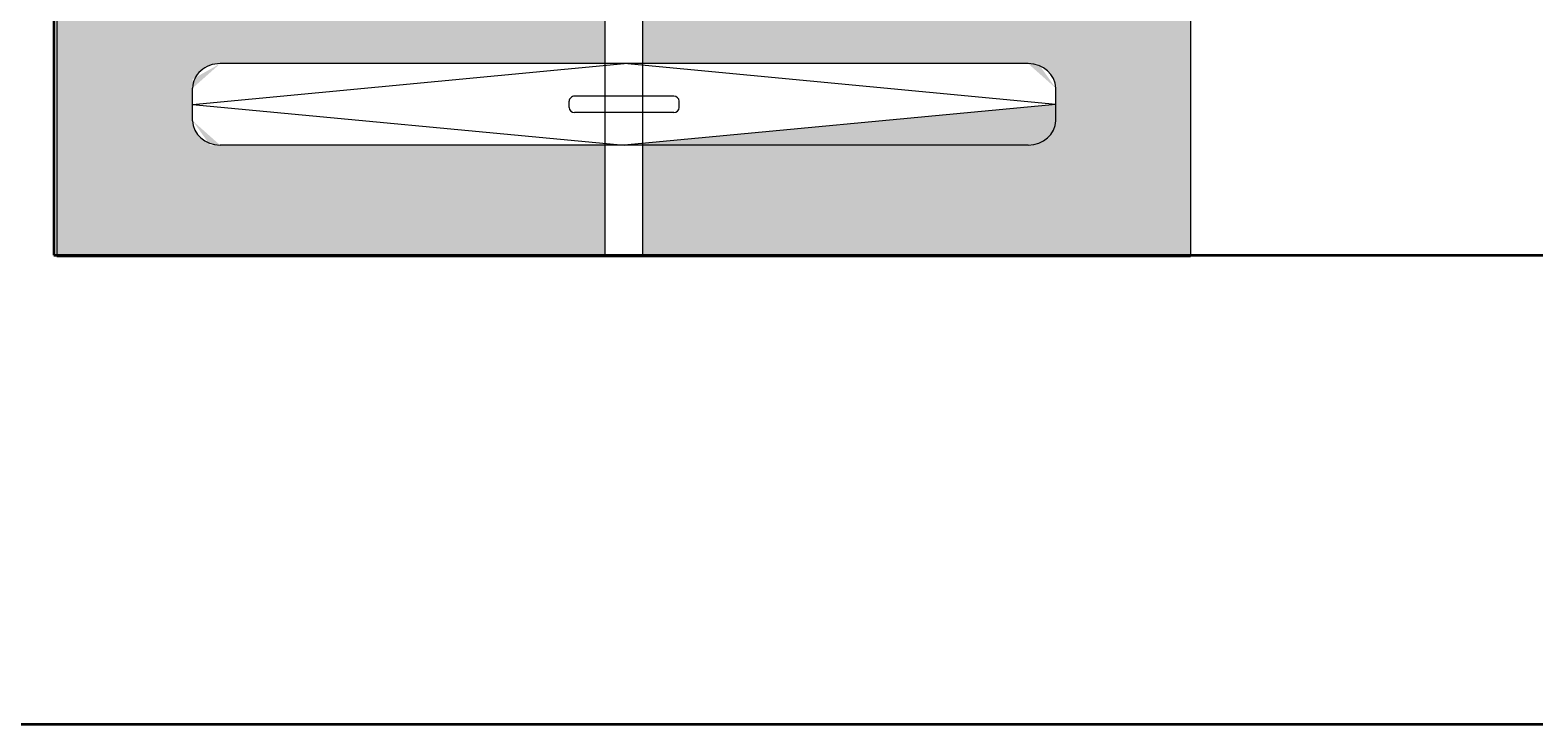
# Model space of a CAD drawing. Units: millimetres. Extents: x 27017497 to 27018854, y 7058029 to 7059154.
# Tile 5 of 91: x 27017622 to 27017651, y 7058133 to 7058146. Entities that reach past the tile are written whole.
import ezdxf

# ---------------------------------------------------------------- set-up
doc = ezdxf.new("R2010")
doc.units = ezdxf.units.MM
for name, color, linetype, lineweight in [('A-ANNO-DIMS', 2, 'Continuous', 18), ('A-FLOR-CASE', 8, 'Continuous', 20), ('A-FLOR-CASE-PATT', 44, 'Continuous', 13), ('A-WALL', 7, 'Continuous', 35)]:
    doc.layers.add(name, color=color, linetype=linetype, lineweight=lineweight)
doc.styles.get("Standard").update_dxf_attribs({"font": 'arial.ttf'})
doc.dimstyles.get("Standard").update_dxf_attribs({"dimtxt": 0.18, "dimasz": 0.18, "dimexe": 0.18, "dimexo": 0.0625, "dimgap": 0.09, "dimtad": 0, "dimtih": 1, "dimtoh": 1, "dimdec": 4, "dimzin": 0, "dimdsep": 46, "dimtxsty": 'Standard', "dimcen": 0.09, "dimadec": 0, "dimazin": 0, "dimtfac": 1, "dimtdec": 4, "dimtofl": 0, "dimtmove": 0, "dimatfit": 3, "dimfxl": 1, "dimtolj": 1, "dimtzin": 0, "dimarcsym": 0})

# ---------------------------------------------------------------- blocks, each defined once
blk = doc.blocks.new('WARDROBE-HANGING')
for p, q in [((0, 21.737), (65.212, 21.737)), ((65.212, 0), (65.212, 21.737)), ((62.293, 19.153), (61.511, 10.877)), ((62.606, 19.153), (61.98, 19.153)), ((62.293, 19.153), (63.076, 10.877)), ((61.511, 18.624), (61.511, 3.13)), ((63.076, 18.624), (63.076, 3.13)), ((62.137, 11.828), (62.137, 9.927)), ((62.356, 11.934), (62.231, 11.934)), ((62.45, 11.828), (62.45, 9.927)), ((0, 11.231), (65.212, 11.231)), ((62.293, 2.602), (61.511, 10.877)), ((62.293, 2.602), (63.076, 10.877)), ((0, 10.506), (65.212, 10.506)), ((62.356, 9.821), (62.231, 9.821)), ((62.606, 2.602), (61.98, 2.602)), ((0, 0), (65.212, 0))]:
    blk.add_line(p, q)
for centre, major_axis, start_param, end_param in [((61.98, 18.624), (0, 0.528), 0, 1.570796), ((62.606, 18.624), (0, 0.528), 4.712389, 6.283185), ((62.231, 11.828), (0, 0.106), 0, 1.570796), ((62.356, 11.828), (0, 0.106), -1.570796, 0), ((62.231, 9.927), (0, 0.106), 1.570796, 3.141593), ((62.356, 9.927), (0, 0.106), 3.141593, 4.712389), ((61.98, 3.13), (0, 0.528), 1.570796, 3.141593), ((62.606, 3.13), (0, 0.528), 3.141593, 4.712389)]:
    blk.add_ellipse(centre, major_axis=major_axis, ratio=0.888892, start_param=start_param, end_param=end_param)
blk = doc.blocks.new('*D47')
at = {"layer": 'A-ANNO-DIMS', "color": 0, "lineweight": -2, "transparency": 16777216}
for p, q in [((27017561.166, 7058294.35), (27017561.166, 7058028.6)), ((27018790.606, 7058294.35), (27018790.606, 7058028.6)), ((27017561.346, 7058028.78), (27018175.431, 7058028.78)), ((27018790.426, 7058028.78), (27018176.341, 7058028.78))]:
    blk.add_line(p, q, dxfattribs=at)
at = {"layer": 'A-ANNO-DIMS', "color": 0, "transparency": 16777216}
for points in [[(27017561.346, 7058028.81), (27017561.346, 7058028.75), (27017561.166, 7058028.78)], [(27018790.426, 7058028.81), (27018790.426, 7058028.75), (27018790.606, 7058028.78)]]:
    blk.add_solid(points, dxfattribs=at)
at = {"layer": 'Defpoints', "color": 0, "transparency": 16777216}
for p in [(27017561.166, 7058294.412), (27018790.606, 7058294.412), (27018790.606, 7058028.78)]:
    blk.add_point(p, dxfattribs=at)
at = {"layer": 'A-ANNO-DIMS', "color": 0, "transparency": 16777216, "insert": (27018175.886, 7058028.78), "char_height": 0.18, "attachment_point": 5}
blk.add_mtext('\\A1;1229.4', dxfattribs=at)
blk = doc.blocks.new('*D48')
at = {"layer": 'A-ANNO-DIMS', "color": 0, "lineweight": -2, "transparency": 16777216}
for p, q in [((27018463.498, 7058622.912), (27017497.536, 7058622.912)), ((27017497.716, 7058622.732), (27017497.716, 7058357.753)), ((27017497.716, 7058092.41), (27017497.716, 7058357.389)), ((27018555.129, 7058092.23), (27017497.536, 7058092.23))]:
    blk.add_line(p, q, dxfattribs=at)
at = {"layer": 'A-ANNO-DIMS', "color": 0, "transparency": 16777216}
for points in [[(27017497.686, 7058622.732), (27017497.746, 7058622.732), (27017497.716, 7058622.912)], [(27017497.686, 7058092.41), (27017497.746, 7058092.41), (27017497.716, 7058092.23)]]:
    blk.add_solid(points, dxfattribs=at)
at = {"layer": 'Defpoints', "color": 0, "transparency": 16777216}
for p in [(27018463.561, 7058622.912), (27017497.716, 7058092.23), (27018555.192, 7058092.23)]:
    blk.add_point(p, dxfattribs=at)
at = {"layer": 'A-ANNO-DIMS', "color": 0, "transparency": 16777216, "insert": (27017497.716, 7058357.571), "char_height": 0.18, "attachment_point": 5}
blk.add_mtext('\\A1;530.7', dxfattribs=at)

msp = doc.modelspace()

# ---------------------------------------------------------------- hatches: boundary and pattern name
at = {"layer": 'A-FLOR-CASE-PATT'}
h = msp.add_hatch(color=256, dxfattribs=at)
h.dxf.hatch_style = 1
edge = h.paths.add_edge_path()
edge.add_line((27017644.461, 7058207.1), (27017639.716, 7058207.1))
edge.add_line((27017639.716, 7058207.1), (27017639.716, 7058207.055))
edge.add_line((27017639.716, 7058207.055), (27017633.955, 7058207.055))
edge.add_line((27017633.955, 7058207.055), (27017633.955, 7058203.02))
edge.add_line((27017633.955, 7058203.02), (27017641.542, 7058203.02))
edge.add_ellipse((27017641.349, 7058202.551), major_axis=(0.528, 0), ratio=0.888892, start_angle=0, end_angle=90, ccw=False)
edge.add_line((27017641.877, 7058202.551), (27017641.877, 7058202.238))
edge.add_line((27017641.877, 7058202.238), (27017633.955, 7058201.488))
edge.add_line((27017633.955, 7058201.488), (27017633.955, 7058199.747))
edge.add_line((27017633.955, 7058199.747), (27017641.542, 7058199.747))
edge.add_ellipse((27017641.349, 7058199.277), major_axis=(0.528, 0), ratio=0.888892, start_angle=0, end_angle=90, ccw=False)
edge.add_line((27017641.877, 7058199.277), (27017641.877, 7058198.964))
edge.add_line((27017641.877, 7058198.964), (27017633.955, 7058198.215))
edge.add_line((27017633.955, 7058198.215), (27017633.955, 7058193.415))
edge.add_line((27017633.955, 7058193.415), (27017641.403, 7058190.704))
edge.add_ellipse((27017641.06, 7058190.329), major_axis=(0.496, -0.181), ratio=0.888892, start_angle=0, end_angle=90, ccw=False)
edge.add_line((27017641.557, 7058190.148), (27017641.45, 7058189.854))
edge.add_line((27017641.45, 7058189.854), (27017633.955, 7058191.806))
edge.add_line((27017633.955, 7058191.806), (27017633.955, 7058188.22))
edge.add_line((27017633.955, 7058188.22), (27017641.542, 7058188.22))
edge.add_ellipse((27017641.349, 7058187.75), major_axis=(0.528, 0), ratio=0.888892, start_angle=0, end_angle=90, ccw=False)
edge.add_line((27017641.877, 7058187.75), (27017641.877, 7058187.437))
edge.add_line((27017641.877, 7058187.437), (27017633.955, 7058186.688))
edge.add_line((27017633.955, 7058186.688), (27017633.955, 7058181.982))
edge.add_line((27017633.955, 7058181.982), (27017641.542, 7058181.982))
edge.add_ellipse((27017641.349, 7058181.513), major_axis=(0.528, 0), ratio=0.888892, start_angle=0, end_angle=90, ccw=False)
edge.add_line((27017641.877, 7058181.513), (27017641.877, 7058181.199))
edge.add_line((27017641.877, 7058181.199), (27017633.955, 7058180.45))
edge.add_line((27017633.955, 7058180.45), (27017633.955, 7058178.709))
edge.add_line((27017633.955, 7058178.709), (27017641.542, 7058178.709))
edge.add_ellipse((27017641.349, 7058178.239), major_axis=(0.528, 0), ratio=0.888892, start_angle=0, end_angle=90, ccw=False)
edge.add_line((27017641.877, 7058178.239), (27017641.877, 7058177.926))
edge.add_line((27017641.877, 7058177.926), (27017633.955, 7058177.177))
edge.add_line((27017633.955, 7058177.177), (27017633.955, 7058173.878))
edge.add_line((27017633.955, 7058173.878), (27017641.403, 7058171.167))
edge.add_ellipse((27017641.06, 7058170.792), major_axis=(0.496, -0.181), ratio=0.888892, start_angle=0, end_angle=90, ccw=False)
edge.add_line((27017641.557, 7058170.611), (27017641.45, 7058170.317))
edge.add_line((27017641.45, 7058170.317), (27017633.955, 7058172.269))
edge.add_line((27017633.955, 7058172.269), (27017633.955, 7058168.293))
edge.add_line((27017633.955, 7058168.293), (27017641.542, 7058168.293))
edge.add_ellipse((27017641.349, 7058167.824), major_axis=(0.528, 0), ratio=0.888892, start_angle=0, end_angle=90, ccw=False)
edge.add_line((27017641.877, 7058167.824), (27017641.877, 7058167.511))
edge.add_line((27017641.877, 7058167.511), (27017633.955, 7058166.762))
edge.add_line((27017633.955, 7058166.762), (27017633.955, 7058160.389))
edge.add_line((27017633.955, 7058160.389), (27017641.542, 7058160.389))
edge.add_ellipse((27017641.349, 7058159.92), major_axis=(0.528, 0), ratio=0.888892, start_angle=0, end_angle=90, ccw=False)
edge.add_line((27017641.877, 7058159.92), (27017641.877, 7058159.607))
edge.add_line((27017641.877, 7058159.607), (27017633.955, 7058158.858))
edge.add_line((27017633.955, 7058158.858), (27017633.955, 7058157.116))
edge.add_line((27017633.955, 7058157.116), (27017641.542, 7058157.116))
edge.add_ellipse((27017641.349, 7058156.647), major_axis=(0.528, 0), ratio=0.888892, start_angle=0, end_angle=90, ccw=False)
edge.add_line((27017641.877, 7058156.647), (27017641.877, 7058156.334))
edge.add_line((27017641.877, 7058156.334), (27017633.955, 7058155.585))
edge.add_line((27017633.955, 7058155.585), (27017633.955, 7058150.784))
edge.add_line((27017633.955, 7058150.784), (27017641.403, 7058148.073))
edge.add_ellipse((27017641.06, 7058147.698), major_axis=(0.496, -0.181), ratio=0.888892, start_angle=0, end_angle=90, ccw=False)
edge.add_line((27017641.557, 7058147.517), (27017641.45, 7058147.223))
edge.add_line((27017641.45, 7058147.223), (27017633.955, 7058149.175))
edge.add_line((27017633.955, 7058149.175), (27017633.955, 7058145.589))
edge.add_line((27017633.955, 7058145.589), (27017641.542, 7058145.589))
edge.add_ellipse((27017641.349, 7058145.119), major_axis=(0.528, 0), ratio=0.888892, start_angle=0, end_angle=90, ccw=False)
edge.add_line((27017641.877, 7058145.119), (27017641.877, 7058144.806))
edge.add_line((27017641.877, 7058144.806), (27017633.955, 7058144.057))
edge.add_line((27017633.955, 7058144.057), (27017633.955, 7058141.912))
edge.add_line((27017633.955, 7058141.912), (27017644.461, 7058141.912))
edge.add_line((27017644.461, 7058141.912), (27017644.461, 7058207.1))
edge = h.paths.add_edge_path()
edge.add_ellipse((27017626.287, 7058195.04), major_axis=(0.496, -0.181), ratio=0.888892, start_angle=180, end_angle=270, ccw=False)
edge.add_line((27017625.79, 7058195.22), (27017626.063, 7058195.97))
edge.add_ellipse((27017626.501, 7058195.628), major_axis=(0.496, -0.181), ratio=0.888892, start_angle=90, end_angle=180, ccw=False)
edge.add_line((27017626.661, 7058196.069), (27017633.23, 7058193.678))
edge.add_line((27017633.23, 7058193.678), (27017633.23, 7058198.182))
edge.add_line((27017633.23, 7058198.182), (27017625.661, 7058198.182))
edge.add_ellipse((27017625.854, 7058198.651), major_axis=(0.528, 0), ratio=0.888892, start_angle=180, end_angle=270, ccw=False)
edge.add_line((27017625.326, 7058198.651), (27017625.326, 7058199.449))
edge.add_ellipse((27017625.854, 7058199.277), major_axis=(0.528, 0), ratio=0.888892, start_angle=90, end_angle=180, ccw=False)
edge.add_line((27017625.854, 7058199.747), (27017633.23, 7058199.747))
edge.add_line((27017633.23, 7058199.747), (27017633.23, 7058201.455))
edge.add_line((27017633.23, 7058201.455), (27017625.661, 7058201.455))
edge.add_ellipse((27017625.854, 7058201.924), major_axis=(0.528, 0), ratio=0.888892, start_angle=180, end_angle=270, ccw=False)
edge.add_line((27017625.326, 7058201.924), (27017625.326, 7058202.722))
edge.add_ellipse((27017625.854, 7058202.551), major_axis=(0.528, 0), ratio=0.888892, start_angle=90, end_angle=180, ccw=False)
edge.add_line((27017625.854, 7058203.02), (27017633.23, 7058203.02))
edge.add_line((27017633.23, 7058203.02), (27017633.23, 7058207.055))
edge.add_line((27017633.23, 7058207.055), (27017622.865, 7058207.055))
edge.add_line((27017622.865, 7058207.055), (27017622.865, 7058201.7))
edge.add_line((27017622.865, 7058201.7), (27017622.724, 7058141.912))
edge.add_line((27017622.724, 7058141.912), (27017633.23, 7058141.912))
edge.add_line((27017633.23, 7058141.912), (27017633.23, 7058144.024))
edge.add_line((27017633.23, 7058144.024), (27017625.661, 7058144.024))
edge.add_ellipse((27017625.854, 7058144.493), major_axis=(0.528, 0), ratio=0.888892, start_angle=180, end_angle=270, ccw=False)
edge.add_line((27017625.326, 7058144.493), (27017625.326, 7058145.291))
edge.add_ellipse((27017625.854, 7058145.119), major_axis=(0.528, 0), ratio=0.888892, start_angle=90, end_angle=180, ccw=False)
edge.add_line((27017625.854, 7058145.589), (27017633.23, 7058145.589))
edge.add_line((27017633.23, 7058145.589), (27017633.23, 7058149.382))
edge.add_line((27017633.23, 7058149.382), (27017625.944, 7058152.034))
edge.add_ellipse((27017626.287, 7058152.409), major_axis=(0.496, -0.181), ratio=0.888892, start_angle=180, end_angle=270, ccw=False)
edge.add_line((27017625.79, 7058152.59), (27017626.063, 7058153.34))
edge.add_ellipse((27017626.501, 7058152.997), major_axis=(0.496, -0.181), ratio=0.888892, start_angle=90, end_angle=180, ccw=False)
edge.add_line((27017626.661, 7058153.439), (27017633.23, 7058151.048))
edge.add_line((27017633.23, 7058151.048), (27017633.23, 7058155.551))
edge.add_line((27017633.23, 7058155.551), (27017625.661, 7058155.551))
edge.add_ellipse((27017625.854, 7058156.021), major_axis=(0.528, 0), ratio=0.888892, start_angle=180, end_angle=270, ccw=False)
edge.add_line((27017625.326, 7058156.021), (27017625.326, 7058156.819))
edge.add_ellipse((27017625.854, 7058156.647), major_axis=(0.528, 0), ratio=0.888892, start_angle=90, end_angle=180, ccw=False)
edge.add_line((27017625.854, 7058157.116), (27017633.23, 7058157.116))
edge.add_line((27017633.23, 7058157.116), (27017633.23, 7058158.824))
edge.add_line((27017633.23, 7058158.824), (27017625.661, 7058158.824))
edge.add_ellipse((27017625.854, 7058159.294), major_axis=(0.528, 0), ratio=0.888892, start_angle=180, end_angle=270, ccw=False)
edge.add_line((27017625.326, 7058159.294), (27017625.326, 7058160.092))
edge.add_ellipse((27017625.854, 7058159.92), major_axis=(0.528, 0), ratio=0.888892, start_angle=90, end_angle=180, ccw=False)
edge.add_line((27017625.854, 7058160.389), (27017633.23, 7058160.389))
edge.add_line((27017633.23, 7058160.389), (27017633.23, 7058166.728))
edge.add_line((27017633.23, 7058166.728), (27017625.661, 7058166.728))
edge.add_ellipse((27017625.854, 7058167.198), major_axis=(0.528, 0), ratio=0.888892, start_angle=180, end_angle=270, ccw=False)
edge.add_line((27017625.326, 7058167.198), (27017625.326, 7058167.996))
edge.add_ellipse((27017625.854, 7058167.824), major_axis=(0.528, 0), ratio=0.888892, start_angle=90, end_angle=180, ccw=False)
edge.add_line((27017625.854, 7058168.293), (27017633.23, 7058168.293))
edge.add_line((27017633.23, 7058168.293), (27017633.23, 7058172.476))
edge.add_line((27017633.23, 7058172.476), (27017625.944, 7058175.128))
edge.add_ellipse((27017626.287, 7058175.503), major_axis=(0.496, -0.181), ratio=0.888892, start_angle=180, end_angle=270, ccw=False)
edge.add_line((27017625.79, 7058175.684), (27017626.063, 7058176.433))
edge.add_ellipse((27017626.501, 7058176.091), major_axis=(0.496, -0.181), ratio=0.888892, start_angle=90, end_angle=180, ccw=False)
edge.add_line((27017626.661, 7058176.533), (27017633.23, 7058174.142))
edge.add_line((27017633.23, 7058174.142), (27017633.23, 7058177.144))
edge.add_line((27017633.23, 7058177.144), (27017625.661, 7058177.144))
edge.add_ellipse((27017625.854, 7058177.613), major_axis=(0.528, 0), ratio=0.888892, start_angle=180, end_angle=270, ccw=False)
edge.add_line((27017625.326, 7058177.613), (27017625.326, 7058178.411))
edge.add_ellipse((27017625.854, 7058178.239), major_axis=(0.528, 0), ratio=0.888892, start_angle=90, end_angle=180, ccw=False)
edge.add_line((27017625.854, 7058178.709), (27017633.23, 7058178.709))
edge.add_line((27017633.23, 7058178.709), (27017633.23, 7058180.417))
edge.add_line((27017633.23, 7058180.417), (27017625.661, 7058180.417))
edge.add_ellipse((27017625.854, 7058180.886), major_axis=(0.528, 0), ratio=0.888892, start_angle=180, end_angle=270, ccw=False)
edge.add_line((27017625.326, 7058180.886), (27017625.326, 7058181.684))
edge.add_ellipse((27017625.854, 7058181.513), major_axis=(0.528, 0), ratio=0.888892, start_angle=90, end_angle=180, ccw=False)
edge.add_line((27017625.854, 7058181.982), (27017633.23, 7058181.982))
edge.add_line((27017633.23, 7058181.982), (27017633.23, 7058186.655))
edge.add_line((27017633.23, 7058186.655), (27017625.661, 7058186.655))
edge.add_ellipse((27017625.854, 7058187.124), major_axis=(0.528, 0), ratio=0.888892, start_angle=180, end_angle=270, ccw=False)
edge.add_line((27017625.326, 7058187.124), (27017625.326, 7058187.922))
edge.add_ellipse((27017625.854, 7058187.75), major_axis=(0.528, 0), ratio=0.888892, start_angle=90, end_angle=180, ccw=False)
edge.add_line((27017625.854, 7058188.22), (27017633.23, 7058188.22))
edge.add_line((27017633.23, 7058188.22), (27017633.23, 7058192.013))
edge.add_line((27017633.23, 7058192.013), (27017625.944, 7058194.665))

# ---------------------------------------------------------------- linework, layer by layer
at = {"layer": 'A-WALL'}
for p, q in [((27017622.666, 7058294.412), (27017622.666, 7058141.912)), ((27017622.666, 7058141.912), (27017802.166, 7058141.912)), ((27017613.666, 7058132.912), (27017802.166, 7058132.912)), ((27017613.666, 7058132.912), (27017802.166, 7058132.912))]:
    msp.add_line(p, q, dxfattribs=at)

# ---------------------------------------------------------------- block references
at = {"layer": 'A-FLOR-CASE', "rotation": 270}
msp.add_blockref('WARDROBE-HANGING', (27017622.724, 7058207.1), dxfattribs=at)

# ---------------------------------------------------------------- dimensions: what is measured, and where the dimension line sits
at = {"layer": 'A-ANNO-DIMS'}
dim = msp.add_linear_dim(base=(27017497.716, 7058092.23), p1=(27018463.561, 7058622.912), p2=(27018555.192, 7058092.23), angle=90, dimstyle='Standard', override={"dimdec": 1, "dimlfac": 1, "dimrnd": 0, "dimzin": 0, "dimdsep": 46, "dimlunit": 2}, dxfattribs=at)
dim.commit()
dim.dimension.update_dxf_attribs({"geometry": '*D48', "text_midpoint": (27017497.716, 7058357.571)})
dim = msp.add_linear_dim(base=(27018790.606, 7058028.78), p1=(27017561.166, 7058294.412), p2=(27018790.606, 7058294.412), dimstyle='Standard', override={"dimdec": 1, "dimlfac": 1, "dimrnd": 0, "dimzin": 0, "dimdsep": 46, "dimlunit": 2}, dxfattribs=at)
dim.commit()
dim.dimension.update_dxf_attribs({"geometry": '*D47', "text_midpoint": (27018175.886, 7058028.78)})

doc.saveas('drawing.dxf')
